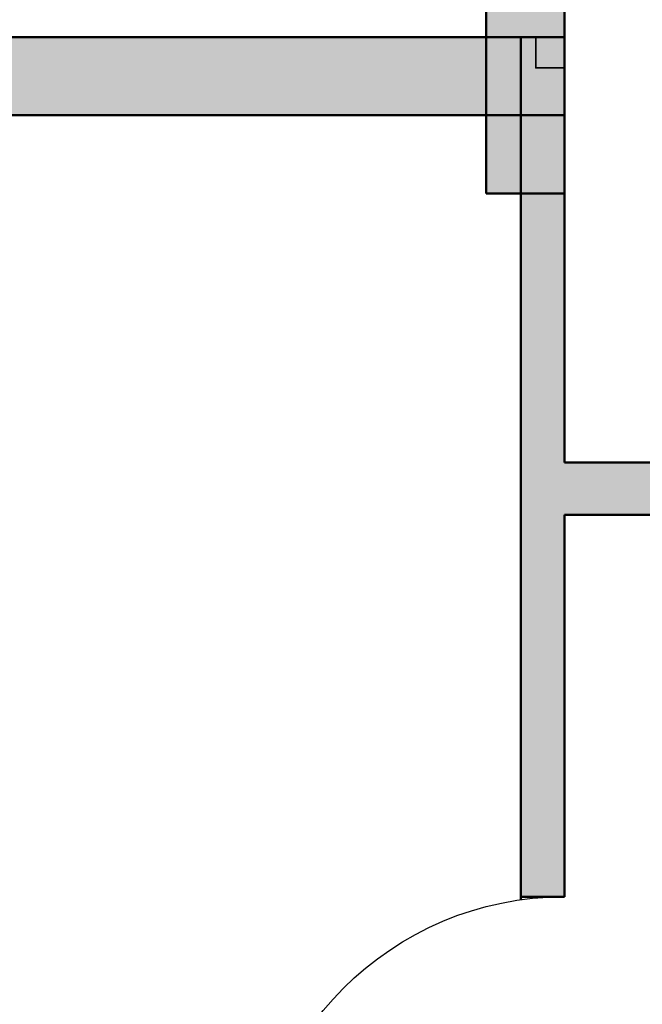
# Model space of a CAD drawing. Units: inches. Extents: x -7 to 1228, y -146 to 1091.
# Tile 80 of 88: x 744 to 816, y 890 to 1003. Entities that reach past the tile are written whole.
import ezdxf

# ---------------------------------------------------------------- set-up
doc = ezdxf.new("R2010")
doc.units = ezdxf.units.IN
for name, color, linetype, lineweight in [('A-COLS', 6, 'Continuous', 35), ('A-DOOR', 4, 'Continuous', 25), ('A-WALL', 7, 'Continuous', 50), ('A-WALL-PATT', 251, 'Continuous', 13)]:
    doc.layers.add(name, color=color, linetype=linetype, lineweight=lineweight)

# ---------------------------------------------------------------- blocks, each defined once
blk = doc.blocks.new('DOOR-900')
blk.add_line((36, 0), (36, 36))
blk.add_arc((36, 0), 36, 90, 180)

msp = doc.modelspace()

# ---------------------------------------------------------------- hatches: boundary and pattern name
at = {"layer": 'A-COLS'}
h = msp.add_hatch(color=256, dxfattribs=at)
h.dxf.hatch_style = 1
h.paths.add_polyline_path([(807, 997.45), (803.71, 997.45), (803.71, 1001), (798, 1001), (798, 983), (807, 983)])
h = msp.add_hatch(color=256, dxfattribs=at)
h.dxf.hatch_style = 1
h.paths.add_polyline_path([(807, 997.45), (807, 1001), (803.71, 1001), (803.71, 997.45)])
at = {"layer": 'A-WALL-PATT'}
h = msp.add_hatch(color=256, dxfattribs=at)
h.dxf.hatch_style = 1
h.paths.add_polyline_path([(69, 568), (60, 568), (60, 493), (63.29, 493), (69, 493)])
h.paths.add_polyline_path([(69, 662.41), (60, 662.41), (60, 586), (69, 586)], flags=17)
h.paths.add_polyline_path([(69, 723), (184, 723), (184, 734), (179, 734), (179, 728), (69, 728), (69, 741.62), (60, 741.62), (60, 698.41), (69, 698.41)], flags=17)
h.paths.add_polyline_path([(69, 782), (231, 782), (231, 728), (231, 723), (231, 586), (236, 586), (236, 787), (69, 787), (69, 800.13), (60, 800.13), (60, 765.62), (69, 765.62)])
h.paths.add_polyline_path([(184, 842), (189, 842), (189, 848), (173, 848), (173, 842), (179, 842), (179, 787), (184, 787)])
h.paths.add_polyline_path([(118.22, 69), (69, 69), (69, 60), (118.22, 60)])
h.paths.add_polyline_path([(227, 69), (154.22, 69), (154.22, 60), (227, 60)])
h.paths.add_polyline_path([(236, 60), (232.71, 60), (227, 60), (227, 36), (236, 36)])
h.paths.add_polyline_path([(389, 60), (380, 60), (380, 36), (389, 36)])
h.paths.add_polyline_path([(384, 181), (380, 181), (380, 115), (380, 78), (384, 78)])
h.paths.add_polyline_path([(380, 115), (334.55, 115), (334.55, 109), (380, 109)])
h.paths.add_polyline_path([(274.55, 115), (236, 115), (236, 201), (232.71, 201), (231, 201), (231, 78), (236, 78), (236, 109), (274.55, 109)])
h.paths.add_polyline_path([(69, 123), (60, 123), (60, 78), (69, 78)])
h.paths.add_polyline_path([(69, 201), (60, 201), (60, 159), (69, 159)])
h.paths.add_polyline_path([(143, 219), (69, 219), (69, 213), (143, 213)], flags=17)
h.paths.add_polyline_path([(189, 219), (184, 219), (184, 274), (231, 274), (231, 219), (236, 219), (236, 279), (184, 279), (184, 297), (179, 297), (179, 279), (69, 279), (69, 290.91), (60, 290.91), (60, 262.18), (69, 262.18), (69, 274), (179, 274), (179, 219), (173, 219), (173, 213), (189, 213)])
h.paths.add_polyline_path([(69, 238.18), (60, 238.18), (60, 219), (69, 219)], flags=17)
h.paths.add_polyline_path([(69, 333), (60, 333), (60, 314.91), (69, 314.91), (69, 316.96)])
h.paths.add_polyline_path([(190, 338), (184, 338), (69, 338), (69, 333), (179, 333), (179, 327), (184, 327), (184, 333.02), (190, 333.05)])
h.paths.add_polyline_path([(69, 386.81), (60, 386.81), (60, 351), (69, 351)])
h.paths.add_polyline_path([(69, 475), (60, 475), (60, 422.81), (69, 422.81)])
h.paths.add_polyline_path([(236, 475), (231, 475), (231, 351.24), (236, 351.24)])
h.paths.add_polyline_path([(384, 475), (380, 475), (380, 362), (384, 362)])
h.paths.add_polyline_path([(547, 307), (439, 307), (439, 356), (445, 356), (445, 362), (433, 362), (433, 307), (380, 307), (380, 244), (380, 241), (384, 241), (384, 301), (433, 301), (433, 277), (439, 277), (439, 301), (547, 301)])
h.paths.add_polyline_path([(547, 241), (439, 241), (439, 247), (433, 247), (433, 235), (547, 235)])
h.paths.add_polyline_path([(450, 69), (440.29, 69), (424.89, 69), (389, 69), (389, 60), (450, 60)])
h.paths.add_polyline_path([(547, 69), (486, 69), (486, 60), (547, 60)])
h.paths.add_polyline_path([(556, 148.27), (547, 148.27), (547, 78), (556, 78)])
h.paths.add_polyline_path([(556, 223), (547, 223), (547, 195), (547, 184.27), (556, 184.27)])
h.paths.add_polyline_path([(556, 311.19), (547, 311.19), (547, 273.08), (556, 273.08)])
h.paths.add_polyline_path([(556, 344), (552.71, 344), (547, 344), (547, 335.19), (556, 335.19)])
h.paths.add_polyline_path([(556, 249.08), (547, 249.08), (547, 241), (556, 241)])
h.paths.add_polyline_path([(547, 362), (475, 362), (475, 356), (547, 356)], flags=0)
h.paths.add_polyline_path([(556, 399.62), (547, 399.62), (547, 362), (556, 362)])
h.paths.add_polyline_path([(556, 475), (547, 475), (547, 435.62), (556, 435.62)])
h.paths.add_polyline_path([(547, 493), (389, 493), (389, 487), (547, 487)])
h.paths.add_polyline_path([(380, 493), (278, 493), (278, 487), (380, 487)])
h.paths.add_polyline_path([(227, 493), (69, 493), (69, 487), (227, 487)])
h.paths.add_polyline_path([(643, 122.44), (634, 122.44), (634, 78), (643, 78)])
h.paths.add_polyline_path([(702.5, 69), (692.79, 69), (677.39, 69), (643, 69), (643, 60), (702.5, 60)])
h.paths.add_polyline_path([(798, 69), (738.5, 69), (738.5, 60), (798, 60)])
h.paths.add_polyline_path([(807, 60), (803.71, 60), (798, 60), (798, 36), (807, 36)])
h.paths.add_polyline_path([(807, 109), (846.75, 109), (846.75, 115), (807, 115), (807, 159), (802, 159), (802, 78), (807, 78)])
h.paths.add_polyline_path([(807, 201), (802, 201), (802, 195), (807, 195)])
h.paths.add_polyline_path([(643, 201), (634, 201), (634, 158.44), (643, 158.44)])
h.paths.add_polyline_path([(756, 225), (751, 225), (751, 219), (643, 219), (643, 213), (756, 213)])
h.paths.add_polyline_path([(643, 240.85), (634, 240.85), (634, 219), (643, 219)])
h.paths.add_polyline_path([(643, 274), (643, 288.63), (634, 288.63), (634, 264.85), (643, 264.85)])
h.paths.add_polyline_path([(802, 279), (756, 279), (756, 297), (751, 297), (751, 279), (643, 279), (643, 274), (751, 274), (751, 255), (756, 255), (756, 274), (802, 274)])
h.paths.add_polyline_path([(807, 333), (803.71, 333), (802, 333), (802, 279), (802, 274), (802, 219), (807, 219)])
h.paths.add_polyline_path([(956, 182), (951, 182), (951, 115), (906.75, 115), (906.75, 109), (951, 109), (951, 78), (956, 78)])
h.paths.add_polyline_path([(960, 60), (951, 60), (951, 36), (960, 36)])
h.paths.add_polyline_path([(1021, 69), (1005.78, 69), (960, 69), (960, 60), (1021, 60)])
h.paths.add_polyline_path([(956, 224), (951, 224), (951, 218), (956, 218)])
h.paths.add_polyline_path([(956, 302), (1004, 302), (1004, 278), (1010, 278), (1010, 302), (1118, 302), (1118, 290.81), (1127, 290.81), (1127, 326.97), (1118, 326.97), (1118, 320.97), (1118, 307), (1010, 307), (1010, 356), (1016, 356), (1016, 362), (1004, 362), (1004, 307), (951, 307), (951, 244), (951, 242), (954.29, 242), (956, 242)])
h.paths.add_polyline_path([(643, 333), (634, 333), (634, 312.63), (643, 312.63), (643, 316.96)])
h.paths.add_polyline_path([(756, 338), (643, 338), (643, 333), (751, 333), (751, 327), (756, 327)])
h.paths.add_polyline_path([(643, 388), (634, 388), (634, 351), (643, 351)])
h.paths.add_polyline_path([(807, 357), (802, 357), (802, 351), (807, 351)])
h.paths.add_polyline_path([(807, 475), (802, 475), (802, 393), (807, 393)])
h.paths.add_polyline_path([(643, 475), (634, 475), (634, 424), (643, 424)])
h.paths.add_polyline_path([(798, 493), (643, 493), (643, 487), (798, 487)])
h.paths.add_polyline_path([(634, 493), (556, 493), (556, 487), (634, 487)])
h.paths.add_polyline_path([(813, 493), (807, 493), (807, 487), (813, 487)])
h.paths.add_polyline_path([(951, 493), (849, 493), (849, 487), (951, 487)])
h.paths.add_polyline_path([(956, 484), (951, 484), (951, 374), (956, 374)])
h.paths.add_polyline_path([(1109, 493), (969, 493), (969, 487), (1109, 487)])
h.paths.add_polyline_path([(1127, 484), (1118, 484), (1118, 450.64), (1127, 450.64)])
h.paths.add_polyline_path([(1127, 414.64), (1118, 414.64), (1118, 365), (1127, 365)])
h.paths.add_polyline_path([(1109, 362), (1046, 362), (1046, 356), (1109, 356)], flags=17)
h.paths.add_polyline_path([(1127, 356), (1123.45, 356), (1118, 356), (1118, 350.97), (1127, 350.97)], flags=0)
h.paths.add_polyline_path([(1127, 266.81), (1118, 266.81), (1118, 262.36), (1118, 242), (1127, 242)], flags=17)
h.paths.add_polyline_path([(1118, 242), (1010, 242), (1010, 248), (1004, 248), (1004, 237), (1118, 237)])
h.paths.add_polyline_path([(1127, 224), (1118, 224), (1118, 170), (1127, 170)])
h.paths.add_polyline_path([(1127, 134), (1118, 134), (1118, 78), (1127, 78)])
h.paths.add_polyline_path([(1118, 69), (1057, 69), (1057, 60), (1118, 60)])
h.paths.add_polyline_path([(227, 571.55), (227, 574), (69, 574), (69, 568), (227, 568)])
h.paths.add_polyline_path([(380, 571.55), (380, 574), (278, 574), (278, 568), (380, 568)])
h.paths.add_polyline_path([(242, 574), (236, 574), (236, 568), (242, 568)])
h.paths.add_polyline_path([(547, 571.55), (547, 574), (389, 574), (389, 568), (547, 568)])
h.paths.add_polyline_path([(384, 733), (380, 733), (380, 586), (384, 586)])
h.paths.add_polyline_path([(556, 646), (634, 646), (634, 655), (547, 655), (547, 586), (556, 586)])
h.paths.add_polyline_path([(634, 574), (556, 574), (556, 568), (634, 568)])
h.paths.add_polyline_path([(643, 655), (634, 655), (634, 586), (643, 586)])
h.paths.add_polyline_path([(798, 574), (643, 574), (643, 568), (798, 568)])
h.paths.add_polyline_path([(643, 663.85), (634, 663.85), (634, 655), (643, 655)])
h.paths.add_polyline_path([(556, 676.97), (547, 676.97), (547, 655), (556, 655)])
h.paths.add_polyline_path([(556, 733), (547, 733), (547, 712.97), (556, 712.97)])
h.paths.add_polyline_path([(643, 710), (634, 710), (634, 699.85), (643, 699.85)])
h.paths.add_polyline_path([(807, 668), (802, 668), (802, 586), (807, 586)])
h.paths.add_polyline_path([(951, 574), (849, 574), (849, 568), (951, 568)])
h.paths.add_polyline_path([(956, 691), (951, 691), (951, 577), (956, 577)])
h.paths.add_polyline_path([(1109, 574), (969, 574), (969, 568), (1109, 568)])
h.paths.add_polyline_path([(1127, 643.4), (1118, 643.4), (1118, 577), (1127, 577)])
h.paths.add_polyline_path([(1127, 568), (1123.45, 568), (1118, 568), (1118, 493), (1127, 493)])
h.paths.add_polyline_path([(1127, 733), (1118, 733), (1118, 679.4), (1127, 679.4)])
h.paths.add_polyline_path([(1127, 777.35), (1118, 777.35), (1118, 770.04), (1118, 751), (1127, 751)], flags=17)
h.paths.add_polyline_path([(1118, 751), (1010, 751), (1010, 757), (1004, 757), (1004, 745), (1118, 745)])
h.paths.add_polyline_path([(956, 811), (1004, 811), (1004, 787), (1010, 787), (1010, 811), (1017.87, 811), (1017.87, 811.63, -0.414214), (1018.25, 812), (1031.98, 812, -0.414214), (1032.35, 811.63), (1032.35, 811), (1118, 811), (1118, 801.35), (1127, 801.35), (1127, 834.69), (1118, 834.69), (1118, 830.24), (1118, 817), (1010, 817), (1010, 866), (1016, 866), (1016, 872), (1004, 872), (1004, 817), (956, 817), (956, 866), (951, 866), (951, 751), (954.29, 751), (956, 751)])
h.paths.add_polyline_path([(1118, 872), (1046, 872), (1046, 866), (1118, 866)], flags=17)
h.paths.add_polyline_path([(1127, 924.71), (1118, 924.71), (1118, 884), (1127, 884)])
h.paths.add_polyline_path([(1127, 866), (1123.71, 866), (1118, 866), (1118, 858.69), (1127, 858.69)], flags=17)
h.paths.add_polyline_path([(956, 983), (951, 983), (951, 952), (807, 952), (807, 983), (802, 983), (802, 902), (807, 902), (807, 946), (951, 946), (951, 884), (956, 884)])
h.paths.add_polyline_path([(807, 842), (802, 842), (802, 787), (756, 787), (756, 806), (751, 806), (751, 787), (643, 787), (643, 782), (751, 782), (751, 764), (756, 764), (756, 782), (802, 782), (802, 728), (807, 728)])
h.paths.add_polyline_path([(756, 848), (643, 848), (643, 842), (751, 842), (751, 836), (756, 836)])
h.paths.add_polyline_path([(756, 734), (751, 734), (751, 728), (643, 728), (643, 723), (756, 723)])
h.paths.add_polyline_path([(643, 749.79), (634, 749.79), (634, 728), (637.29, 728), (643, 728)])
h.paths.add_polyline_path([(643, 805.41), (634, 805.41), (634, 773.79), (643, 773.79)])
h.paths.add_polyline_path([(643, 896.66), (634, 896.66), (634, 860), (637.29, 860), (643, 860)])
h.paths.add_polyline_path([(643, 842), (634, 842), (634, 829.41), (643, 829.41)])
h.paths.add_polyline_path([(643, 983), (634, 983), (634, 932.66), (643, 932.66)])
h.paths.add_polyline_path([(1127, 983), (1118, 983), (1118, 960.71), (1127, 960.71)])
h.paths.add_polyline_path([(1118, 1001), (1077.53, 1001), (1077.53, 992), (1118, 992)])
h.paths.add_polyline_path([(1041.53, 1001), (960, 1001), (960, 992), (1041.53, 992)])
h.paths.add_polyline_path([(960, 1025), (951, 1025), (951, 1001), (954.29, 1001), (960, 1001)])
h.paths.add_polyline_path([(807, 1025), (798, 1025), (798, 1001), (807, 1001)])
h.paths.add_polyline_path([(798, 1001), (738.5, 1001), (738.5, 992), (798, 992)])
h.paths.add_polyline_path([(702.5, 1001), (643, 1001), (643, 992), (702.5, 992)])
h.paths.add_polyline_path([(547, 1001), (499.11, 1001), (499.11, 992), (547, 992)])
h.paths.add_polyline_path([(463.11, 1001), (389, 1001), (389, 992), (463.11, 992)])
h.paths.add_polyline_path([(389, 1025), (380, 1025), (380, 1022), (380, 1001), (383.29, 1001), (389, 1001)])
h.paths.add_polyline_path([(236, 1025), (227, 1025), (227, 1001), (236, 1001)])
h.paths.add_polyline_path([(236, 983), (231, 983), (231, 860), (236, 860)])
h.paths.add_polyline_path([(274.55, 952), (236, 952), (236, 946), (274.55, 946)])
h.paths.add_polyline_path([(380, 952), (334.55, 952), (334.55, 946), (380, 946)])
h.paths.add_polyline_path([(384, 983), (380, 983), (380, 884), (383.29, 884), (384, 884)])
h.paths.add_polyline_path([(227, 1001), (155.01, 1001), (155.01, 992), (162.87, 992), (227, 992)])
h.paths.add_polyline_path([(119.01, 1001), (69, 1001), (69, 992), (119.01, 992)])
h.paths.add_polyline_path([(69, 983), (60, 983), (60, 922.99), (69, 922.99)])
h.paths.add_polyline_path([(69, 886.99), (60, 886.99), (60, 860), (63.29, 860), (69, 860)])
h.paths.add_polyline_path([(143, 848), (69, 848), (69, 842), (143, 842)])

# ---------------------------------------------------------------- linework, layer by layer
at = {"layer": 'A-COLS'}
msp.add_lwpolyline([(807, 1001), (803.71, 1001), (803.71, 997.45), (807, 997.45)], close=True, dxfattribs=at)
at = {"layer": 'A-WALL'}
for p, q in [((798, 1001), (798, 1025)), ((807, 1025), (807, 1001)), ((807, 1001), (634, 1001)), ((807, 1001), (798, 1001)), ((798, 1001), (798, 983)), ((802, 1001), (802, 902)), ((802, 901.65), (802, 1001)), ((807, 1001), (807, 952)), ((807, 983), (807, 1001)), ((807, 952), (807, 1001)), ((807, 992), (634, 992)), ((798, 983), (807, 983)), ((951, 952), (807, 952)), ((951, 946), (807, 946)), ((807, 946), (807, 902)), ((807, 902), (807, 946)), ((807, 902), (802, 902))]:
    msp.add_line(p, q, dxfattribs=at)

# ---------------------------------------------------------------- block references
at = {"layer": 'A-DOOR', "extrusion": (0, 0, -1), "zscale": -1, "rotation": 269.9999999999997}
msp.add_blockref('DOOR-900', (-807, 902), dxfattribs=at)

doc.saveas('drawing.dxf')
